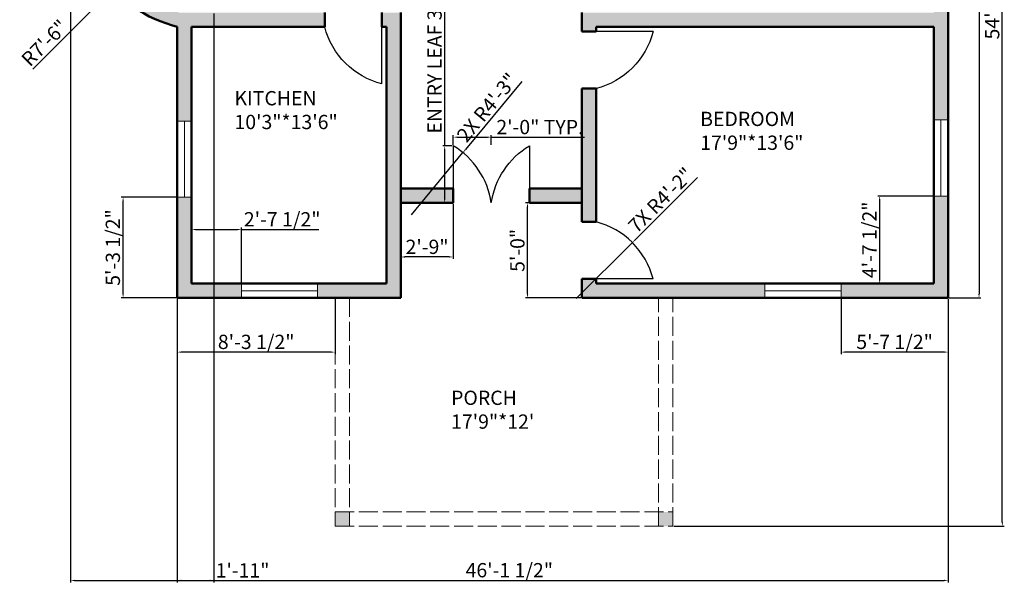
# Model space of a CAD drawing. Units: inches. Extents: x 2291 to 2912, y 1781 to 2517.
# Tile 1 of 2: x 2291 to 2912, y 1781 to 2143. Entities that reach past the tile are written whole.
import ezdxf

# ---------------------------------------------------------------- set-up
doc = ezdxf.new("R2010")
doc.units = ezdxf.units.IN
doc.linetypes.add('ACAD_ISO02W100', pattern=[15, 12, -3])
for name, color, linetype, lineweight in [('A-ANNO-DIMS', 2, 'Continuous', 18), ('A-AREA-IDEN', 7, 'Continuous', 25), ('A-DOOR', 3, 'Continuous', 25), ('A-FLOR-OVHD', 8, 'ACAD_ISO02W100', 18), ('A-GLAZ', 4, 'Continuous', 18), ('A-WALL', 7, 'Continuous', 50)]:
    doc.layers.add(name, color=color, linetype=linetype, lineweight=lineweight)
doc.layers.add('A-WALL-PATT', color=18, linetype='Continuous', lineweight=13, true_color=0x000000)
doc.styles.get("Standard").update_dxf_attribs({"font": 'arial.ttf'})
doc.dimstyles.new('ISO-25', dxfattribs={"dimtxt": 9, "dimasz": 2.5, "dimexe": 1.25, "dimexo": 0.625, "dimtad": 1, "dimlunit": 3, "dimtxsty": 'Standard', "dimcen": 2.5, "dimadec": 0, "dimazin": 0, "dimtfac": 1, "dimtmove": 0, "dimatfit": 3, "dimfxl": 1, "dimarcsym": 0})

# ---------------------------------------------------------------- blocks, each defined once
blk = doc.blocks.new('*D3')
at = {"layer": 'A-ANNO-DIMS', "color": 0, "lineweight": -2, "transparency": 16777216}
for p, q in [((2877.16, 2471.1), (2897.25, 2471.1)), ((2896, 2468.6), (2896, 1969.6)), ((2877.16, 1967.1), (2897.25, 1967.1))]:
    blk.add_line(p, q, dxfattribs=at)
at = {"layer": 'A-ANNO-DIMS', "color": 0, "transparency": 16777216}
for points in [[(2895.58, 2468.6), (2896.42, 2468.6), (2896, 2471.1)], [(2895.58, 1969.6), (2896.42, 1969.6), (2896, 1967.1)]]:
    blk.add_solid(points, dxfattribs=at)
at = {"layer": 'Defpoints', "color": 0, "transparency": 16777216}
for p in [(2876.53, 2471.1), (2876.53, 1967.1), (2896, 1967.1)]:
    blk.add_point(p, dxfattribs=at)
at = {"layer": 'A-ANNO-DIMS', "color": 0, "transparency": 16777216, "insert": (2890.86, 2219.1), "char_height": 9, "attachment_point": 5, "rotation": 90}
blk.add_mtext("42'", dxfattribs=at)
blk = doc.blocks.new('WINDOW-48IN')
for p, q in [((9, 48), (0, 48)), ((0, 48), (0, 0)), ((4.5, 0), (4.5, 48)), ((9, 0), (9, 48)), ((0, 0), (9, 0))]:
    blk.add_line(p, q)
blk = doc.blocks.new('DOOR-SINGLE-36IN')
blk.add_line((36, 36), (36, 0))
blk.add_arc((48.43, -12.43), 50, 104.39819, 165.60181)
blk = doc.blocks.new('DOOR-ENTRY-PAIRED-LEAF')
blk.add_line((0, 36), (0, 0))
blk.add_arc((-26.41, -7.61), 50.98, 8.58016, 58.79997)
blk = doc.blocks.new('*D11')
at = {"layer": 'A-ANNO-DIMS', "color": 0, "lineweight": -2, "transparency": 16777216}
for p, q in [((2559.13, 2063.1), (2559.13, 2202.28)), ((2563.91, 2063.1), (2557.88, 2063.1)), ((2559.13, 2029.6), (2559.13, 2060.6)), ((2563.91, 2027.1), (2557.88, 2027.1))]:
    blk.add_line(p, q, dxfattribs=at)
at = {"layer": 'A-ANNO-DIMS', "color": 0, "transparency": 16777216}
for points in [[(2558.72, 2060.6), (2559.55, 2060.6), (2559.13, 2063.1)], [(2558.72, 2029.6), (2559.55, 2029.6), (2559.13, 2027.1)]]:
    blk.add_solid(points, dxfattribs=at)
at = {"layer": 'Defpoints', "color": 0, "transparency": 16777216}
for p in [(2559.13, 2063.1), (2564.53, 2063.1), (2564.53, 2027.1)]:
    blk.add_point(p, dxfattribs=at)
at = {"layer": 'A-ANNO-DIMS', "color": 0, "transparency": 16777216, "insert": (2553.91, 2133.94), "char_height": 9, "attachment_point": 5, "rotation": 90}
blk.add_mtext('ENTRY LEAF 3\'-0" TYP.', dxfattribs=at)
blk = doc.blocks.new('*D12')
at = {"layer": 'A-ANNO-DIMS', "color": 0, "lineweight": -2, "transparency": 16777216}
for p, q in [((2564.53, 2063.73), (2564.53, 2069.75)), ((2567.03, 2068.5), (2586.03, 2068.5)), ((2588.53, 2063.73), (2588.53, 2069.75)), ((2588.53, 2068.5), (2647.3, 2068.5))]:
    blk.add_line(p, q, dxfattribs=at)
at = {"layer": 'A-ANNO-DIMS', "color": 0, "transparency": 16777216}
for points in [[(2567.03, 2068.92), (2567.03, 2068.08), (2564.53, 2068.5)], [(2586.03, 2068.92), (2586.03, 2068.08), (2588.53, 2068.5)]]:
    blk.add_solid(points, dxfattribs=at)
at = {"layer": 'Defpoints', "color": 0, "transparency": 16777216}
for p in [(2588.53, 2068.5), (2564.53, 2063.1), (2588.53, 2063.1)]:
    blk.add_point(p, dxfattribs=at)
at = {"layer": 'A-ANNO-DIMS', "color": 0, "transparency": 16777216, "insert": (2619.17, 2073.72), "char_height": 9, "attachment_point": 5}
blk.add_mtext('2\'-0" TYP.', dxfattribs=at)
blk = doc.blocks.new('*D13')
at = {"layer": 'A-ANNO-DIMS', "color": 0, "lineweight": -2, "transparency": 16777216}
for p, q in [((2877.16, 2471.1), (2911.95, 2471.1)), ((2910.7, 1825.6), (2910.7, 2468.6)), ((2703.66, 1823.1), (2911.95, 1823.1))]:
    blk.add_line(p, q, dxfattribs=at)
at = {"layer": 'A-ANNO-DIMS', "color": 0, "transparency": 16777216}
for points in [[(2910.28, 2468.6), (2911.12, 2468.6), (2910.7, 2471.1)], [(2910.28, 1825.6), (2911.12, 1825.6), (2910.7, 1823.1)]]:
    blk.add_solid(points, dxfattribs=at)
at = {"layer": 'Defpoints', "color": 0, "transparency": 16777216}
for p in [(2876.53, 2471.1), (2910.7, 2471.1), (2703.03, 1823.1)]:
    blk.add_point(p, dxfattribs=at)
at = {"layer": 'A-ANNO-DIMS', "color": 0, "transparency": 16777216, "insert": (2905.48, 2147.1), "char_height": 9, "attachment_point": 5, "rotation": 90}
blk.add_mtext('54\'-0"', dxfattribs=at)
blk = doc.blocks.new('*D14')
at = {"layer": 'A-ANNO-DIMS', "color": 0, "lineweight": -2, "transparency": 16777216}
for p, q in [((2323.2, 2224.48), (2323.2, 1787.69)), ((2876.53, 1966.48), (2876.53, 1787.69)), ((2325.7, 1788.94), (2874.03, 1788.94))]:
    blk.add_line(p, q, dxfattribs=at)
at = {"layer": 'A-ANNO-DIMS', "color": 0, "transparency": 16777216}
for points in [[(2325.7, 1789.35), (2325.7, 1788.52), (2323.2, 1788.94)], [(2874.03, 1789.35), (2874.03, 1788.52), (2876.53, 1788.94)]]:
    blk.add_solid(points, dxfattribs=at)
at = {"layer": 'Defpoints', "color": 0, "transparency": 16777216}
for p in [(2323.2, 2225.1), (2876.53, 1967.1), (2876.53, 1788.94)]:
    blk.add_point(p, dxfattribs=at)
at = {"layer": 'A-ANNO-DIMS', "color": 0, "transparency": 16777216, "insert": (2599.87, 1794.21), "char_height": 9, "attachment_point": 5}
blk.add_mtext('46\'-1 1/2"', dxfattribs=at)
blk = doc.blocks.new('*D15')
at = {"layer": 'A-ANNO-DIMS', "color": 0, "lineweight": -2, "transparency": 16777216}
for p, q in [((2390.53, 1966.48), (2390.53, 1931.69)), ((2490.03, 1966.48), (2490.03, 1931.69)), ((2487.53, 1932.94), (2393.03, 1932.94))]:
    blk.add_line(p, q, dxfattribs=at)
at = {"layer": 'A-ANNO-DIMS', "color": 0, "transparency": 16777216}
for points in [[(2393.03, 1933.35), (2393.03, 1932.52), (2390.53, 1932.94)], [(2487.53, 1933.35), (2487.53, 1932.52), (2490.03, 1932.94)]]:
    blk.add_solid(points, dxfattribs=at)
at = {"layer": 'Defpoints', "color": 0, "transparency": 16777216}
for p in [(2390.53, 1967.1), (2490.03, 1967.1), (2390.53, 1932.94)]:
    blk.add_point(p, dxfattribs=at)
at = {"layer": 'A-ANNO-DIMS', "color": 0, "transparency": 16777216, "insert": (2440.28, 1938.22), "char_height": 9, "attachment_point": 5}
blk.add_mtext('8\'-3 1/2"', dxfattribs=at)
blk = doc.blocks.new('*D16')
at = {"layer": 'A-ANNO-DIMS', "color": 0, "lineweight": -2, "transparency": 16777216}
for p, q in [((2644.91, 2027.1), (2610.12, 2027.1)), ((2611.37, 1969.6), (2611.37, 2024.6)), ((2644.91, 1967.1), (2610.12, 1967.1))]:
    blk.add_line(p, q, dxfattribs=at)
at = {"layer": 'A-ANNO-DIMS', "color": 0, "transparency": 16777216}
for points in [[(2610.95, 2024.6), (2611.79, 2024.6), (2611.37, 2027.1)], [(2610.95, 1969.6), (2611.79, 1969.6), (2611.37, 1967.1)]]:
    blk.add_solid(points, dxfattribs=at)
at = {"layer": 'Defpoints', "color": 0, "transparency": 16777216}
for p in [(2611.37, 2027.1), (2645.53, 2027.1), (2645.53, 1967.1)]:
    blk.add_point(p, dxfattribs=at)
at = {"layer": 'A-ANNO-DIMS', "color": 0, "transparency": 16777216, "insert": (2606.15, 1997.1), "char_height": 9, "attachment_point": 5, "rotation": 90}
blk.add_mtext('5\'-0"', dxfattribs=at)
blk = doc.blocks.new('*D21')
at = {"layer": 'A-ANNO-DIMS', "color": 0, "lineweight": -2, "transparency": 16777216}
for p, q in [((2399.53, 1976.73), (2399.53, 2011.52)), ((2431.03, 1976.73), (2431.03, 2011.52)), ((2402.03, 2010.27), (2428.53, 2010.27)), ((2431.03, 2010.27), (2479.83, 2010.27))]:
    blk.add_line(p, q, dxfattribs=at)
at = {"layer": 'A-ANNO-DIMS', "color": 0, "transparency": 16777216}
for points in [[(2402.03, 2010.68), (2402.03, 2009.85), (2399.53, 2010.27)], [(2428.53, 2010.68), (2428.53, 2009.85), (2431.03, 2010.27)]]:
    blk.add_solid(points, dxfattribs=at)
at = {"layer": 'Defpoints', "color": 0, "transparency": 16777216}
for p in [(2431.03, 2010.27), (2399.53, 1976.1), (2431.03, 1976.1)]:
    blk.add_point(p, dxfattribs=at)
at = {"layer": 'A-ANNO-DIMS', "color": 0, "transparency": 16777216, "insert": (2456.68, 2015.54), "char_height": 9, "attachment_point": 5}
blk.add_mtext('2\'-7 1/2"', dxfattribs=at)
blk = doc.blocks.new('*D22')
at = {"layer": 'A-ANNO-DIMS', "color": 0, "lineweight": -2, "transparency": 16777216}
for p, q in [((2809.03, 1966.48), (2809.03, 1931.69)), ((2876.53, 1966.48), (2876.53, 1931.69)), ((2874.03, 1932.94), (2811.53, 1932.94))]:
    blk.add_line(p, q, dxfattribs=at)
at = {"layer": 'A-ANNO-DIMS', "color": 0, "transparency": 16777216}
for points in [[(2811.53, 1933.35), (2811.53, 1932.52), (2809.03, 1932.94)], [(2874.03, 1933.35), (2874.03, 1932.52), (2876.53, 1932.94)]]:
    blk.add_solid(points, dxfattribs=at)
at = {"layer": 'Defpoints', "color": 0, "transparency": 16777216}
for p in [(2809.03, 1967.1), (2876.53, 1967.1), (2809.03, 1932.94)]:
    blk.add_point(p, dxfattribs=at)
at = {"layer": 'A-ANNO-DIMS', "color": 0, "transparency": 16777216, "insert": (2842.78, 1938.21), "char_height": 9, "attachment_point": 5}
blk.add_mtext('5\'-7 1/2"', dxfattribs=at)
blk = doc.blocks.new('*D25')
at = {"layer": 'A-ANNO-DIMS', "color": 0, "lineweight": -2, "transparency": 16777216}
for p, q in [((2866.91, 2031.37), (2832.12, 2031.37)), ((2833.37, 1978.6), (2833.37, 2028.87)), ((2866.91, 1976.1), (2832.12, 1976.1))]:
    blk.add_line(p, q, dxfattribs=at)
at = {"layer": 'A-ANNO-DIMS', "color": 0, "transparency": 16777216}
for points in [[(2832.95, 2028.87), (2833.79, 2028.87), (2833.37, 2031.37)], [(2832.95, 1978.6), (2833.79, 1978.6), (2833.37, 1976.1)]]:
    blk.add_solid(points, dxfattribs=at)
at = {"layer": 'Defpoints', "color": 0, "transparency": 16777216}
for p in [(2833.37, 2031.37), (2867.53, 2031.37), (2867.53, 1976.1)]:
    blk.add_point(p, dxfattribs=at)
at = {"layer": 'A-ANNO-DIMS', "color": 0, "transparency": 16777216, "insert": (2828.09, 2003.74), "char_height": 9, "attachment_point": 5, "rotation": 90}
blk.add_mtext('4\'-7 1/2"', dxfattribs=at)
blk = doc.blocks.new('*D26')
at = {"layer": 'A-ANNO-DIMS', "color": 0, "lineweight": -2, "transparency": 16777216}
for p, q in [((2389.91, 2030.7), (2355.12, 2030.7)), ((2356.37, 1969.6), (2356.37, 2028.2)), ((2389.91, 1967.1), (2355.12, 1967.1))]:
    blk.add_line(p, q, dxfattribs=at)
at = {"layer": 'A-ANNO-DIMS', "color": 0, "transparency": 16777216}
for points in [[(2355.95, 2028.2), (2356.79, 2028.2), (2356.37, 2030.7)], [(2355.95, 1969.6), (2356.79, 1969.6), (2356.37, 1967.1)]]:
    blk.add_solid(points, dxfattribs=at)
at = {"layer": 'Defpoints', "color": 0, "transparency": 16777216}
for p in [(2356.37, 2030.7), (2390.53, 2030.7), (2390.53, 1967.1)]:
    blk.add_point(p, dxfattribs=at)
at = {"layer": 'A-ANNO-DIMS', "color": 0, "transparency": 16777216, "insert": (2351.09, 1998.9), "char_height": 9, "attachment_point": 5, "rotation": 90}
blk.add_mtext('5\'-3 1/2"', dxfattribs=at)
blk = doc.blocks.new('*D30')
at = {"layer": 'A-ANNO-DIMS', "color": 0, "lineweight": -2, "transparency": 16777216}
for p, q in [((2531.53, 2026.48), (2531.53, 1991.69)), ((2564.53, 2026.48), (2564.53, 1991.69)), ((2562.03, 1992.94), (2534.03, 1992.94))]:
    blk.add_line(p, q, dxfattribs=at)
at = {"layer": 'A-ANNO-DIMS', "color": 0, "transparency": 16777216}
for points in [[(2534.03, 1993.35), (2534.03, 1992.52), (2531.53, 1992.94)], [(2562.03, 1993.35), (2562.03, 1992.52), (2564.53, 1992.94)]]:
    blk.add_solid(points, dxfattribs=at)
at = {"layer": 'Defpoints', "color": 0, "transparency": 16777216}
for p in [(2531.53, 2027.1), (2564.53, 2027.1), (2531.53, 1992.94)]:
    blk.add_point(p, dxfattribs=at)
at = {"layer": 'A-ANNO-DIMS', "color": 0, "transparency": 16777216, "insert": (2548.03, 1998.16), "char_height": 9, "attachment_point": 5}
blk.add_mtext('2\'-9"', dxfattribs=at)
blk = doc.blocks.new('*D36')
at = {"layer": 'A-ANNO-DIMS', "color": 0, "lineweight": -2, "transparency": 16777216}
for p, q in [((2413.53, 2146.48), (2413.53, 1787.69)), ((2390.53, 2137.48), (2390.53, 1787.69)), ((2393.03, 1788.94), (2411.03, 1788.94)), ((2413.53, 1788.94), (2447.35, 1788.94))]:
    blk.add_line(p, q, dxfattribs=at)
at = {"layer": 'A-ANNO-DIMS', "color": 0, "transparency": 16777216}
for points in [[(2393.03, 1789.35), (2393.03, 1788.52), (2390.53, 1788.94)], [(2411.03, 1789.35), (2411.03, 1788.52), (2413.53, 1788.94)]]:
    blk.add_solid(points, dxfattribs=at)
at = {"layer": 'Defpoints', "color": 0, "transparency": 16777216}
for p in [(2413.53, 2147.1), (2390.53, 2138.1), (2413.53, 1788.94)]:
    blk.add_point(p, dxfattribs=at)
at = {"layer": 'A-ANNO-DIMS', "color": 0, "transparency": 16777216, "insert": (2431.69, 1794.08), "char_height": 9, "attachment_point": 5}
blk.add_mtext('1\'-11"', dxfattribs=at)
blk = doc.blocks.new('*D37')
at = {"layer": 'A-ANNO-DIMS', "color": 0, "lineweight": -2, "transparency": 16777216}
for p, q in [((2413.08, 2225.1), (2349.53, 2161.55)), ((2299.46, 2111.47), (2347.76, 2159.78))]:
    blk.add_line(p, q, dxfattribs=at)
at = {"layer": 'A-ANNO-DIMS', "color": 0, "transparency": 16777216}
blk.add_solid([(2347.47, 2160.08), (2348.06, 2159.49), (2349.53, 2161.55)], dxfattribs=at)
at = {"layer": 'Defpoints', "color": 0, "transparency": 16777216}
for p in [(2413.08, 2225.1), (2349.53, 2161.55)]:
    blk.add_point(p, dxfattribs=at)
at = {"layer": 'A-ANNO-DIMS', "color": 0, "transparency": 16777216, "insert": (2307.71, 2127.11), "char_height": 9, "attachment_point": 5, "rotation": 45.00141}
blk.add_mtext('R7\'-6"', dxfattribs=at)
blk = doc.blocks.new('*D40')
at = {"layer": 'A-ANNO-DIMS', "color": 0, "lineweight": -2, "transparency": 16777216}
for p, q in [((2607.8, 2103.65), (2572.23, 2060.69)), ((2538.13, 2019.5), (2570.64, 2058.76))]:
    blk.add_line(p, q, dxfattribs=at)
at = {"layer": 'A-ANNO-DIMS', "color": 0, "transparency": 16777216}
blk.add_solid([(2571.91, 2060.95), (2572.55, 2060.42), (2570.64, 2058.76)], dxfattribs=at)
at = {"layer": 'Defpoints', "color": 0, "transparency": 16777216}
for p in [(2570.64, 2058.76), (2538.13, 2019.5)]:
    blk.add_point(p, dxfattribs=at)
at = {"layer": 'A-ANNO-DIMS', "color": 0, "transparency": 16777216, "insert": (2586.79, 2086.47), "char_height": 9, "attachment_point": 5, "rotation": 50.37818}
blk.add_mtext('2X R4\'-3"', dxfattribs=at)
blk = doc.blocks.new('*D41')
at = {"layer": 'A-ANNO-DIMS', "color": 0, "lineweight": -2, "transparency": 16777216}
for p, q in [((2718.51, 2043.08), (2679.23, 2003.79)), ((2642.1, 1966.67), (2677.46, 2002.03))]:
    blk.add_line(p, q, dxfattribs=at)
at = {"layer": 'A-ANNO-DIMS', "color": 0, "transparency": 16777216}
blk.add_solid([(2678.93, 2004.09), (2679.52, 2003.5), (2677.46, 2002.03)], dxfattribs=at)
at = {"layer": 'Defpoints', "color": 0, "transparency": 16777216}
for p in [(2677.46, 2002.03), (2642.1, 1966.67)]:
    blk.add_point(p, dxfattribs=at)
at = {"layer": 'A-ANNO-DIMS', "color": 0, "transparency": 16777216, "insert": (2696.11, 2027.96), "char_height": 9, "attachment_point": 5, "rotation": 45.00014}
blk.add_mtext('7X R4\'-2"', dxfattribs=at)

msp = doc.modelspace()

# ---------------------------------------------------------------- hatches: boundary and pattern name
at = {"layer": 'A-WALL-PATT'}
h = msp.add_hatch(color=256, dxfattribs=at)
h.dxf.hatch_style = 1
h.paths.add_polyline_path([(2608.229, 2471.101), (2500.749, 2471.101), (2500.749, 2462.101), (2574.534, 2462.101), (2574.534, 2312.101), (2571.534, 2312.101), (2571.534, 2303.101), (2666.534, 2303.101), (2666.534, 2312.101), (2583.534, 2312.101), (2583.534, 2462.101), (2608.229, 2462.101)])
h.paths.add_polyline_path([(2452.749, 2471.101), (2390.534, 2471.101), (2390.534, 2416.836), (2399.534, 2416.836), (2399.534, 2462.101), (2452.749, 2462.101)])
h.paths.add_polyline_path([(2399.534, 2368.836), (2390.534, 2368.836), (2390.534, 2312.101, 0.7738955), (2390.534, 2138.101), (2390.534, 2078.695), (2399.534, 2078.695), (2399.534, 2138.101), (2483.534, 2138.101), (2483.534, 2147.101), (2391.712, 2147.101, -0.7629082), (2391.712, 2303.101), (2535.534, 2303.101), (2535.534, 2312.101), (2399.534, 2312.101)])
h.paths.add_polyline_path([(2714.534, 2462.101), (2766.881, 2462.101), (2766.881, 2471.101), (2705.534, 2471.101), (2705.534, 2312.101), (2702.534, 2312.101), (2702.534, 2303.101), (2717.534, 2303.101), (2717.534, 2312.101), (2714.534, 2312.101)])
h.paths.add_polyline_path([(2876.534, 2471.101), (2814.881, 2471.101), (2814.881, 2462.101), (2867.534, 2462.101), (2867.534, 2419.508), (2876.534, 2419.508)])
h.paths.add_polyline_path([(2876.534, 2371.508), (2867.534, 2371.508), (2867.534, 2312.101), (2753.534, 2312.101), (2753.534, 2303.101), (2867.534, 2303.101), (2867.534, 2300.101), (2876.534, 2300.101)])
h.paths.add_polyline_path([(2876.534, 2264.101), (2867.534, 2264.101), (2867.534, 2225.473), (2876.534, 2225.473)])
h.paths.add_polyline_path([(2876.534, 2177.473), (2867.534, 2177.473), (2867.534, 2147.101), (2645.534, 2147.101), (2645.534, 2135.101), (2654.534, 2135.101), (2654.534, 2138.101), (2867.534, 2138.101), (2867.534, 2079.372), (2876.534, 2079.372)])
h.paths.add_polyline_path([(2531.534, 2147.101), (2519.534, 2147.101), (2519.534, 2138.101), (2522.534, 2138.101), (2522.534, 1976.101), (2479.032, 1976.101), (2479.032, 1967.101), (2531.534, 1967.101)])
h.paths.add_polyline_path([(2399.534, 2030.695), (2390.534, 2030.695), (2390.534, 1967.101), (2431.032, 1967.101), (2431.032, 1976.101), (2399.534, 1976.101)])
h.paths.add_polyline_path([(2654.534, 2099.101), (2645.534, 2099.101), (2645.534, 2015.101), (2654.534, 2015.101)])
h.paths.add_polyline_path([(2761.034, 1976.101), (2654.534, 1976.101), (2654.534, 1979.101), (2645.534, 1979.101), (2645.534, 1967.101), (2761.034, 1967.101)])
h.paths.add_polyline_path([(2876.534, 2031.372), (2867.534, 2031.372), (2867.534, 1976.101), (2809.034, 1976.101), (2809.034, 1967.101), (2876.534, 1967.101)])
h.paths.add_polyline_path([(2499.035, 1832.101), (2490.035, 1832.101), (2490.035, 1823.101), (2499.035, 1823.101)])
h.paths.add_polyline_path([(2703.035, 1832.101), (2694.035, 1832.101), (2694.035, 1823.101), (2703.035, 1823.101)])
h = msp.add_hatch(color=256, dxfattribs=at)
h.dxf.hatch_style = 1
h.paths.add_polyline_path([(2645.534, 2036.101), (2612.534, 2036.101), (2612.534, 2027.101), (2645.534, 2027.101)])
h.paths.add_polyline_path([(2564.534, 2036.101), (2531.534, 2036.101), (2531.534, 2027.101), (2564.534, 2027.101)])

# ---------------------------------------------------------------- linework, layer by layer
at = {"layer": 'A-FLOR-OVHD'}
for p, q in [((2490.035, 1967.101), (2490.035, 1823.101)), ((2499.035, 1967.101), (2499.035, 1823.101)), ((2694.035, 1823.101), (2694.035, 1967.101)), ((2703.035, 1823.101), (2703.035, 1967.101)), ((2490.035, 1832.101), (2703.035, 1832.101)), ((2490.035, 1823.101), (2703.035, 1823.101))]:
    msp.add_line(p, q, dxfattribs=at)
at = {"layer": 'A-WALL'}
for p, q in [((2876.534, 1967.101), (2876.534, 2264.101)), ((2483.534, 2138.101), (2483.534, 2147.101)), ((2519.534, 2138.101), (2519.534, 2147.101)), ((2531.534, 2147.101), (2531.534, 1967.101)), ((2645.534, 2135.101), (2645.534, 2147.101)), ((2390.534, 2138.101), (2390.534, 1967.101)), ((2399.534, 2138.101), (2399.534, 1976.101)), ((2483.534, 2138.101), (2399.534, 2138.101)), ((2522.534, 2138.101), (2519.534, 2138.101)), ((2522.534, 2138.101), (2519.534, 2138.101)), ((2522.534, 2138.101), (2522.534, 1976.101)), ((2867.534, 2138.101), (2654.534, 2138.101)), ((2654.534, 2138.101), (2654.534, 2135.101)), ((2654.534, 2135.101), (2654.534, 2138.101)), ((2867.534, 1976.101), (2867.534, 2138.101)), ((2654.534, 2135.101), (2645.534, 2135.101)), ((2654.534, 2099.101), (2645.534, 2099.101)), ((2645.534, 2015.101), (2645.534, 2099.101)), ((2654.534, 2015.101), (2654.534, 2099.101)), ((2564.534, 2036.101), (2531.534, 2036.101)), ((2564.534, 2027.101), (2564.534, 2036.101)), ((2645.534, 2036.101), (2612.534, 2036.101)), ((2612.534, 2027.101), (2612.534, 2036.101)), ((2564.534, 2027.101), (2531.534, 2027.101)), ((2645.534, 2027.101), (2612.534, 2027.101)), ((2645.534, 2015.101), (2645.534, 2027.101)), ((2654.534, 2015.101), (2645.534, 2015.101)), ((2399.534, 1976.101), (2522.534, 1976.101)), ((2645.534, 1967.101), (2645.534, 1979.101)), ((2654.534, 1979.101), (2645.534, 1979.101)), ((2654.534, 1976.101), (2654.534, 1979.101)), ((2654.534, 1976.101), (2654.534, 1979.101)), ((2654.534, 1976.101), (2867.534, 1976.101)), ((2390.534, 1967.101), (2531.534, 1967.101)), ((2645.534, 1967.101), (2876.534, 1967.101))]:
    msp.add_line(p, q, dxfattribs=at)
msp.add_arc((2413.078, 2225.101), 89.874, 104.52775, 255.47225, dxfattribs=at)

# ---------------------------------------------------------------- block references
at = {"layer": 'A-DOOR', "extrusion": (0, 0, -1), "zscale": -1}
for p, rotation in [((-2483.534, 2138.102), 180), ((-2654.533, 2099.102), 90.00000000000044)]:
    msp.add_blockref('DOOR-SINGLE-36IN', p, dxfattribs=dict(at, rotation=rotation))
at = {"layer": 'A-DOOR'}
msp.add_blockref('DOOR-ENTRY-PAIRED-LEAF', (2564.534, 2027.101), dxfattribs=at)
at = {"layer": 'A-DOOR', "extrusion": (0, 0, -1), "zscale": -1}
msp.add_blockref('DOOR-ENTRY-PAIRED-LEAF', (-2612.533, 2027.101), dxfattribs=at)
at = {"layer": 'A-DOOR', "rotation": 270.0000000000063}
msp.add_blockref('DOOR-SINGLE-36IN', (2654.533, 2015.101), dxfattribs=at)
at = {"layer": 'A-GLAZ'}
for p, rotation in [((2399.533, 2078.695), 180), ((2876.533, 2079.372), 180), ((2431.033, 1976.101), 270.0000000000014), ((2761.034, 1976.101), 270.0000000000012)]:
    msp.add_blockref('WINDOW-48IN', p, dxfattribs=dict(at, rotation=rotation))

# ---------------------------------------------------------------- texts
at = {"layer": 'A-AREA-IDEN', "char_height": 9, "attachment_point": 1}
for s, width, insert in [('KITCHEN\\P10\'3"*13\'6"', 62.25917, (2426.597, 2097.579)), ('BEDROOM\\P17\'9"*13\'6"', 65.58771, (2720.217, 2084.509)), ('PORCH\\P17\'9"*12\'', 115.71017, (2563.171, 1908.609))]:
    msp.add_mtext_dynamic_manual_height_columns(s, width=width, gutter_width=12.5, heights=[0], dxfattribs=dict(at, insert=insert))

# ---------------------------------------------------------------- dimensions: what is measured, and where the dimension line sits
at = {"layer": 'A-ANNO-DIMS'}
for base, p1, p2, angle, override, picture, middle in [((2910.699, 2471.101), (2703.035, 1823.101), (2876.534, 2471.101), 90, {"dimdec": 1, "dimlfac": 1, "dimrnd": 0, "dimzin": 1, "dimdsep": 46, "dimlunit": 4, "dimfrac": 2}, '*D13', (2905.479, 2147.101)), ((2896, 1967.101), (2876.534, 2471.101), (2876.534, 1967.101), 90, {"dimclrd": 0, "dimclre": 0, "dimclrt": 0}, '*D3', (2890.857, 2219.101)), ((2356.369, 2030.695), (2390.534, 1967.101), (2390.534, 2030.695), 90, {"dimdec": 1, "dimlfac": 1, "dimrnd": 0, "dimzin": 1, "dimdsep": 46, "dimlunit": 4, "dimfrac": 2}, '*D26', (2351.087, 1998.898)), ((2833.369, 2031.372), (2867.534, 1976.101), (2867.534, 2031.372), 90, {"dimdec": 1, "dimlfac": 1, "dimrnd": 0, "dimzin": 1, "dimdsep": 46, "dimlunit": 4, "dimfrac": 2}, '*D25', (2828.09, 2003.737)), ((2531.534, 1992.936), (2564.534, 2027.101), (2531.534, 2027.101), 180, {"dimdec": 1, "dimlfac": 1, "dimrnd": 0, "dimzin": 1, "dimdsep": 46, "dimlunit": 4, "dimfrac": 2}, '*D30', (2548.034, 1998.157)), ((2611.369, 2027.101), (2645.534, 1967.101), (2645.534, 2027.101), 90, {"dimdec": 1, "dimlfac": 1, "dimrnd": 0, "dimzin": 1, "dimdsep": 46, "dimlunit": 4, "dimfrac": 2}, '*D16', (2606.149, 1997.101)), ((2390.534, 1932.936), (2490.035, 1967.101), (2390.534, 1967.101), 180, {"dimdec": 1, "dimlfac": 1, "dimrnd": 0, "dimzin": 1, "dimdsep": 46, "dimlunit": 4, "dimfrac": 2}, '*D15', (2440.284, 1938.218)), ((2809.034, 1932.936), (2876.534, 1967.101), (2809.034, 1967.101), 180, {"dimdec": 1, "dimlfac": 1, "dimrnd": 0, "dimzin": 1, "dimdsep": 46, "dimlunit": 4, "dimfrac": 2}, '*D22', (2842.784, 1938.215))]:
    dim = msp.add_linear_dim(base=base, p1=p1, p2=p2, angle=angle, dimstyle='ISO-25', override=override, dxfattribs=at)
    dim.commit()
    dim.dimension.update_dxf_attribs({"geometry": picture, "text_midpoint": middle})
dim = msp.add_radius_dim(center=(2413.078, 2225.101), mpoint=(2349.53, 2161.55), dimstyle='ISO-25', override={"dimdec": 1, "dimlfac": 1, "dimrnd": 0, "dimzin": 1, "dimdsep": 46, "dimlunit": 4, "dimfrac": 2}, dxfattribs=at)
dim.commit()
dim.dimension.update_dxf_attribs({"geometry": '*D37', "text_midpoint": (2311.401, 2123.419), "dimtype": 164})
for base, p1, p2, picture, middle in [((2876.534, 1788.936), (2323.205, 2225.101), (2876.534, 1967.101), '*D14', (2599.869, 1794.215)), ((2413.534, 1788.936), (2390.534, 2138.101), (2413.534, 2147.101), '*D36', (2431.693, 1794.08)), ((2431.032, 2010.266), (2399.534, 1976.101), (2431.032, 1976.101), '*D21', (2456.682, 2015.545))]:
    dim = msp.add_linear_dim(base=base, p1=p1, p2=p2, dimstyle='ISO-25', override={"dimdec": 1, "dimlfac": 1, "dimrnd": 0, "dimzin": 1, "dimdsep": 46, "dimlunit": 4, "dimfrac": 2}, dxfattribs=at)
    dim.commit()
    dim.dimension.update_dxf_attribs({"geometry": picture, "text_midpoint": middle})
dim = msp.add_linear_dim(base=(2559.134, 2063.101), p1=(2564.534, 2027.101), p2=(2564.534, 2063.101), angle=90, text='ENTRY LEAF <> TYP.', dimstyle='ISO-25', override={"dimdec": 1, "dimlfac": 1, "dimrnd": 0, "dimzin": 1, "dimdsep": 46, "dimlunit": 4, "dimfrac": 2}, dxfattribs=at)
dim.commit()
dim.dimension.update_dxf_attribs({"geometry": '*D11', "text_midpoint": (2553.91, 2133.941)})
for center, mpoint, text, picture, middle in [((2538.125, 2019.496), (2570.635, 2058.764), '2X <>', '*D40', (2586.789, 2086.466)), ((2642.1, 1966.667), (2677.458, 2002.026), '7X <>', '*D41', (2696.111, 2027.958))]:
    dim = msp.add_radius_dim(center=center, mpoint=mpoint, text=text, dimstyle='ISO-25', override={"dimdec": 1, "dimlfac": 1, "dimrnd": 0, "dimzin": 1, "dimdsep": 46, "dimlunit": 4, "dimfrac": 2}, dxfattribs=at)
    dim.commit()
    dim.dimension.update_dxf_attribs({"geometry": picture, "text_midpoint": middle})
dim = msp.add_linear_dim(base=(2588.534, 2068.501), p1=(2564.534, 2063.101), p2=(2588.534, 2063.101), text='<> TYP.', dimstyle='ISO-25', override={"dimdec": 1, "dimlfac": 1, "dimrnd": 0, "dimzin": 1, "dimdsep": 46, "dimlunit": 4, "dimfrac": 2}, dxfattribs=at)
dim.commit()
dim.dimension.update_dxf_attribs({"geometry": '*D12', "text_midpoint": (2619.165, 2073.722)})

doc.saveas('drawing.dxf')
